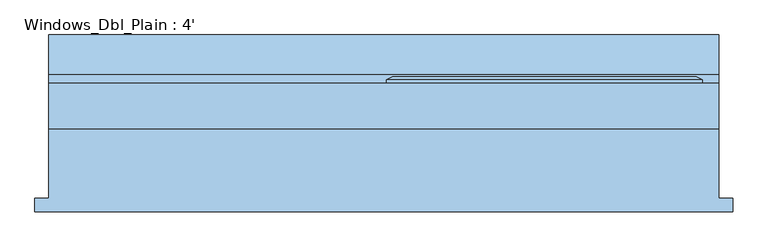
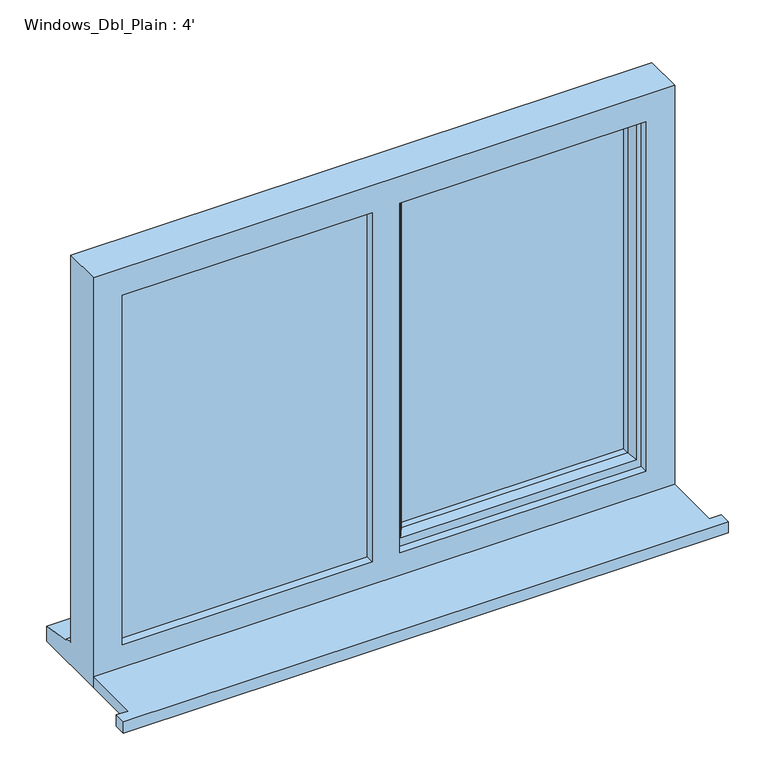
"""IFC4 building model written with IfcOpenShell, lengths in millimetres: window geometry, Windows_Dbl_Plain : 4'."""

from ifc_helpers import new_model, si_unit, frame, origin, place, context, project, spatial, polyline, outline, extrude, faceted_brep, source, transform, mapped, element, save


def windows_dbl_plain_4_0a19b8d2(model_context):
    return source(origin(), model_context, "Body", "SolidModel", [
        extrude(outline(polyline([(-919.6, -146.0834322), (-919.6, -121.0834322), (-894.6, -121.0834322), (-894.6, 4.9965678), (324.6, 4.9965678), (324.6, -121.0834322), (349.6, -121.0834322), (349.6, -146.0834322), (-919.6, -146.0834322)])), frame((0.0, 0.0, 1200.0), z_axis=(0.0, 0.0, 1.0), x_axis=(1.0, 0.0, 0.0)), (0.0, 0.0, 1.0), 25.0),
        faceted_brep([(-280.0, 87.9965678, 2080.0), (-280.0, 93.7700705, 2080.0), (-280.0, 93.7700705, 1253.0), (-280.0, 87.9965678, 1253.0), (-270.0, 22.9965678, 2070.0), (-270.0, 87.9965678, 2070.0), (-270.0, 87.9965678, 1263.0), (-270.0, 22.9965678, 1263.0), (-230.0, 37.4894677, 2030.0), (-240.1480377, 22.9965678, 2040.1480377), (-240.1480377, 22.9965678, 1292.8519623), (-230.0, 37.4894677, 1303.0), (-230.0, 51.9965678, 2030.0), (-230.0, 51.9965678, 1303.0), (-240.0, 75.9965678, 2040.0), (-240.0, 51.9965678, 2040.0), (-240.0, 51.9965678, 1293.0), (-240.0, 75.9965678, 1293.0), (-230.0, 93.7700705, 2030.0), (-230.0, 75.9965678, 2030.0), (-230.0, 75.9965678, 1303.0), (-230.0, 93.7700705, 1303.0), (-247.4457548, 99.5435732, 2047.4457548), (-247.4457548, 99.5435732, 1285.5542452), (-269.2153903, 99.5435732, 2069.2153903), (-269.2153903, 99.5435732, 1263.7846097), (294.6, 93.7700705, 1253.0), (294.6, 87.9965678, 1253.0), (284.6, 87.9965678, 1263.0), (284.6, 22.9965678, 1263.0), (254.7480377, 22.9965678, 1292.8519623), (244.6, 37.4894677, 1303.0), (244.6, 51.9965678, 1303.0), (254.6, 51.9965678, 1293.0), (254.6, 75.9965678, 1293.0), (244.6, 75.9965678, 1303.0), (244.6, 93.7700705, 1303.0), (262.0457548, 99.5435732, 1285.5542452), (283.8153903, 99.5435732, 1263.7846097), (294.6, 93.7700705, 2080.0), (294.6, 87.9965678, 2080.0), (284.6, 87.9965678, 2070.0), (284.6, 22.9965678, 2070.0), (254.7480377, 22.9965678, 2040.1480377), (244.6, 37.4894677, 2030.0), (244.6, 51.9965678, 2030.0), (254.6, 51.9965678, 2040.0), (254.6, 75.9965678, 2040.0), (244.6, 75.9965678, 2030.0), (244.6, 93.7700705, 2030.0), (262.0457548, 99.5435732, 2047.4457548), (283.8153903, 99.5435732, 2069.2153903)], [[[0, 1, 2, 3]], [[4, 5, 6, 7]], [[8, 9, 10, 11]], [[12, 8, 11, 13]], [[14, 15, 16, 17]], [[18, 19, 20, 21]], [[22, 18, 21, 23]], [[1, 24, 25, 2]], [[3, 2, 26, 27]], [[7, 6, 28, 29]], [[11, 10, 30, 31]], [[13, 11, 31, 32]], [[17, 16, 33, 34]], [[21, 20, 35, 36]], [[23, 21, 36, 37]], [[2, 25, 38, 26]], [[27, 26, 39, 40]], [[29, 28, 41, 42]], [[31, 30, 43, 44]], [[32, 31, 44, 45]], [[34, 33, 46, 47]], [[36, 35, 48, 49]], [[37, 36, 49, 50]], [[26, 38, 51, 39]], [[40, 39, 1, 0]], [[3, 27, 40, 0], [5, 41, 28, 6]], [[42, 41, 5, 4]], [[7, 29, 42, 4], [9, 43, 30, 10]], [[44, 43, 9, 8]], [[45, 44, 8, 12]], [[15, 46, 33, 16], [13, 32, 45, 12]], [[47, 46, 15, 14]], [[17, 34, 47, 14], [19, 48, 35, 20]], [[49, 48, 19, 18]], [[50, 49, 18, 22]], [[24, 51, 38, 25], [23, 37, 50, 22]], [[39, 51, 24, 1]]]),
        extrude(outline(polyline([(2050.0, -310.0), (2070.0, -310.0), (2070.0, -854.6), (1263.0, -854.6), (1263.0, -310.0), (1283.0, -310.0), (1283.0, -834.6), (2050.0, -834.6), (2050.0, -310.0)])), frame((0.0, 46.9965678, 0.0), z_axis=(0.0, 1.0, 0.0), x_axis=(0.0, 0.0, 1.0)), (0.0, 0.0, 1.0), 41.0),
        faceted_brep([(324.6, 4.9965678, 2110.0), (-894.6, 4.9965678, 2110.0), (-894.6, 4.9965678, 1200.0), (324.6, 4.9965678, 1200.0), (264.6, 4.9965678, 2050.0), (264.6, 4.9965678, 1275.0), (-252.0, 4.9965678, 1275.0), (-252.0, 4.9965678, 2050.0), (-310.0, 4.9965678, 2050.0), (-310.0, 4.9965678, 1275.0), (-834.6, 4.9965678, 1275.0), (-834.6, 4.9965678, 2050.0), (-894.6, 87.9965678, 2110.0), (-894.6, 87.9965678, 1251.0), (-894.6, 102.9965678, 1249.68767), (-894.6, 102.9965678, 1244.7449676), (-894.6, 175.4965678, 1233.8088847), (-894.6, 175.4965678, 1200.0), (324.6, 87.9965678, 2110.0), (324.6, 87.9965678, 1251.0), (-854.6, 87.9965678, 2070.0), (-854.6, 87.9965678, 1263.0), (-310.0, 87.9965678, 1263.0), (-310.0, 87.9965678, 2070.0), (-270.0, 87.9965678, 2070.0), (-270.0, 87.9965678, 1263.0), (284.6, 87.9965678, 1263.0), (284.6, 87.9965678, 2070.0), (-854.6, 22.9965678, 2070.0), (-854.6, 22.9965678, 1263.0), (-300.0, 22.9965678, 2070.0), (-300.0, 22.9965678, 1263.0), (-310.0, 22.9965678, 2050.0), (-834.6, 22.9965678, 2050.0), (-834.6, 22.9965678, 1275.0), (-310.0, 22.9965678, 1275.0), (-270.0, 22.9965678, 2070.0), (284.6, 22.9965678, 2070.0), (284.6, 22.9965678, 1263.0), (-270.0, 22.9965678, 1263.0), (264.6, 22.9965678, 2050.0), (-252.0, 22.9965678, 2050.0), (-252.0, 22.9965678, 1275.0), (264.6, 22.9965678, 1275.0), (-310.0, 46.9965678, 2070.0), (-300.0, 46.9965678, 2070.0), (324.6, 175.4965678, 1200.0), (324.6, 175.4965678, 1233.8088847), (324.6, 102.9965678, 1244.7449676), (324.6, 102.9965678, 1249.68767), (-300.0, 46.9965678, 1263.0), (-310.0, 46.9965678, 1263.0)], [[[0, 1, 2, 3], [4, 5, 6, 7], [8, 9, 10, 11]], [[2, 1, 12, 13, 14, 15, 16, 17]], [[13, 12, 18, 19], [20, 21, 22, 23], [24, 25, 26, 27]], [[21, 20, 28, 29]], [[28, 30, 31, 29], [32, 33, 34, 35]], [[36, 37, 38, 39], [40, 41, 42, 43]], [[33, 11, 10, 34]], [[1, 0, 18, 12]], [[28, 20, 23, 44, 45, 30]], [[27, 37, 36, 24]], [[11, 33, 32, 8]], [[40, 4, 7, 41]], [[19, 18, 0, 3, 46, 47, 48, 49]], [[27, 26, 38, 37]], [[4, 40, 43, 5]], [[45, 50, 31, 30]], [[50, 45, 44, 51]], [[51, 44, 23, 22]], [[25, 24, 36, 39]], [[41, 7, 6, 42]], [[8, 32, 35, 9]], [[46, 3, 2, 17]], [[47, 46, 17, 16]], [[48, 47, 16, 15]], [[49, 48, 15, 14]], [[19, 49, 14, 13]], [[22, 21, 29, 31, 50, 51]], [[26, 25, 39, 38]], [[6, 5, 43, 42]], [[35, 34, 10, 9]]]),
        extrude(outline(polyline([(-854.6, 46.9965678), (-300.0, 46.9965678), (-300.0, 22.9965678), (-854.6, 22.9965678), (-854.6, 46.9965678)])), frame((0.0, 0.0, 1263.0), z_axis=(0.0, 0.0, 1.0), x_axis=(1.0, 0.0, 0.0)), (0.0, 0.0, 1.0), 807.0),
        extrude(outline(polyline([(254.6, 51.9965678), (-240.0, 51.9965678), (-240.0, 75.9965678), (254.6, 75.9965678), (254.6, 51.9965678)])), frame((0.0, 0.0, 1293.0), z_axis=(0.0, 0.0, 1.0), x_axis=(1.0, 0.0, 0.0)), (0.0, 0.0, 1.0), 747.0),
    ])


if __name__ == "__main__":
    model = new_model("IFC4")
    model_context = context("Model", 3, world=origin())
    ifc_project = project(units=[si_unit("LENGTHUNIT", "METRE", prefix="MILLI")], contexts=[model_context])
    site = spatial("IfcSite", under=ifc_project)
    building = spatial("IfcBuilding", under=site)
    placement = place(None, origin())
    windows_dbl_plain_4_shape = windows_dbl_plain_4_0a19b8d2(model_context)
    element("IfcWindow", 1, ObjectType="Windows_Dbl_Plain : 4'", at=placement, inside=building, context=model_context, shape_type="MappedRepresentation", body=[
        mapped(windows_dbl_plain_4_shape, transform((0.0, 0.0, 0.0), x_axis=(1.0, 0.0, 0.0), y_axis=(0.0, 1.0, 0.0), z_axis=(0.0, 0.0, 1.0))),
    ])
    save(model, "model.ifc")

# Revit data of these elements
# Type "Windows_Dbl_Plain : 4'"
#   Type Mark = "63"
#   Operation = "DoublePanelVertical"
#   Construction Type Id = "GSP4R"
#   Manufacturer = "Revit"
#   Keynote = "L10"
#   Analytic Construction = "1/8 in Pilkington single glazing"
#   Wrap Layers (Ext) from Ext = 102.5 mm
#   Wrap Layers (Int) from Ext = 177.5 mm
#   Window Board Projection = 25 mm
#   Window Board Extension = 25 mm
#   Visual Light Transmittance = 0.9
#   Solar Heat Gain Coefficient = 0.78
#   Rough Width = 1219.2 mm
#   Rough Height = 910 mm
#   Height = 910 mm
#   Width = 1219.2 mm
#   Heat Transfer Coefficient (U) = 3.6886 W/(m²·K)
#   Glazing Thickness = 24 mm
#   FrameOffset - External = 50 mm
#   Frame Depth = 65 mm
#   Default Head Height = 2110 mm
#   Cill Depth = 87.5 mm
#   Cavity Closer Width = 50 mm
#   Cavity Closer Offset from Ext = 102.5 mm
#   Cavity Closer Depth = 85 mm
#   Vis - Cavity Closers = yes
#   Define Thermal Properties by = 1
#   Material Trim = Window Frame
#   Material Glass = Glass
#   Material Frame = Window Frame
#   Wall Closure = (empty or 0)
# Element 1 (IfcWindow, "Windows_Dbl_Plain : 4'")
#   Materials on its faces: "Window Frame", "Glass"
# Materials
#   "Window Frame": colour RGB 249 249 249, transparency 0, Keynote = "L10", Cost = 0
#   "Glass": class "Glass", colour RGB 0 128 192, transparency 0.9, Description = "Soda Lime Glass", Cost = 0
